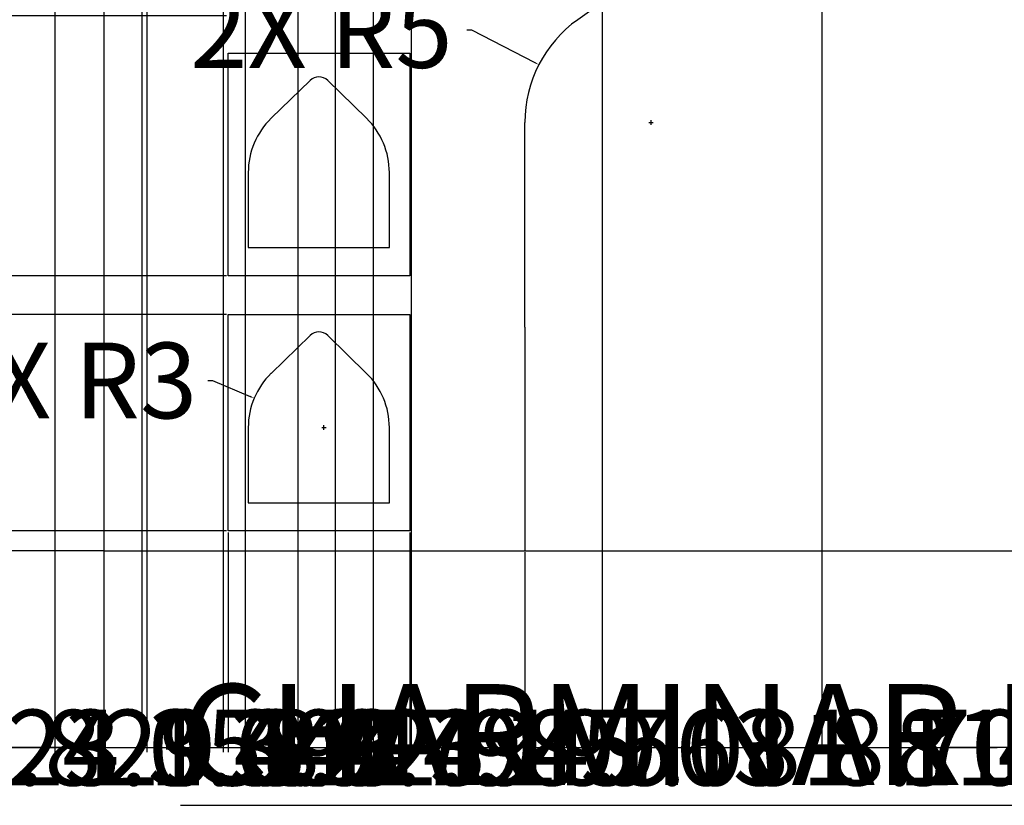
# Model space of a CAD drawing. Units: inches. Extents: x 168 to 318, y 152 to 314.
# Tile 2 of 7: x 201 to 240, y 152 to 183. Entities that reach past the tile are written whole.
import ezdxf

# ---------------------------------------------------------------- set-up
doc = ezdxf.new("R2010")
doc.units = ezdxf.units.IN
doc.header["$MEASUREMENT"] = 0
for name, color, linetype, lineweight in [('A-ANNO-DIMS', 2, 'Continuous', 18), ('A-ANNO-TEXT', 3, 'Continuous', 25), ('A-ELEV', 7, 'Continuous', 25)]:
    doc.layers.add(name, color=color, linetype=linetype, lineweight=lineweight)
doc.styles.get("Standard").update_dxf_attribs({"font": 'arial.ttf'})
doc.dimstyles.get("Standard").update_dxf_attribs({"dimtxt": 3, "dimasz": 0.18, "dimexe": 0.18, "dimexo": 0.0625, "dimgap": 0.09, "dimtad": 0, "dimtih": 1, "dimtoh": 1, "dimdec": 1, "dimzin": 0, "dimdsep": 46, "dimlunit": 3, "dimtxsty": 'Standard', "dimcen": 0.09, "dimadec": 0, "dimazin": 0, "dimtfac": 1, "dimtdec": 1, "dimtofl": 0, "dimtmove": 0, "dimatfit": 3, "dimfxl": 1, "dimtolj": 1, "dimtzin": 0, "dimarcsym": 0})

# ---------------------------------------------------------------- blocks, each defined once
blk = doc.blocks.new('NICHE-ARCHED')
for p, q in [((0.908, 5.124), (2.451, 6.627)), ((3.149, 6.626), (4.687, 5.124)), ((0, 2.975), (0, 0)), ((5.592, 0), (5.592, 2.977)), ((0, 0), (5.592, 0))]:
    blk.add_line(p, q)
for centre, radius, start, end in [((2.8, 6.268), 0.5, 45.6844, 134.2257), ((3, 2.975), 3, 134.2257, 180), ((2.592, 2.977), 3, 0, 45.6844)]:
    blk.add_arc(centre, radius, start, end)
blk = doc.blocks.new('*D29')
at = {"layer": 'A-ANNO-DIMS', "color": 0, "lineweight": -2, "ltscale": 0.2, "transparency": 16777216}
for p, q in [((184.724, 242.139), (184.724, 154.215)), ((299.445, 242.139), (299.445, 154.215)), ((184.904, 154.395), (235.924, 154.395)), ((299.265, 154.395), (248.245, 154.395))]:
    blk.add_line(p, q, dxfattribs=at)
at = {"layer": 'A-ANNO-DIMS', "color": 0, "ltscale": 0.2, "transparency": 16777216}
for points in [[(184.904, 154.425), (184.904, 154.365), (184.724, 154.395)], [(299.265, 154.425), (299.265, 154.365), (299.445, 154.395)]]:
    blk.add_solid(points, dxfattribs=at)
at = {"layer": 'Defpoints', "color": 0, "ltscale": 0.2, "transparency": 16777216}
for p in [(184.724, 242.201), (299.445, 242.201), (299.445, 154.395)]:
    blk.add_point(p, dxfattribs=at)
at = {"layer": 'A-ANNO-DIMS', "color": 0, "ltscale": 0.2, "transparency": 16777216, "insert": (242.084, 154.395), "char_height": 3, "attachment_point": 5}
blk.add_mtext('\\A1;114.72', dxfattribs=at)
blk = doc.blocks.new('*D48')
at = {"layer": 'A-ANNO-DIMS', "color": 0, "lineweight": -2, "ltscale": 0.2, "transparency": 16777216}
for p, q in [((192.404, 162.133), (192.404, 154.215)), ((204.404, 162.133), (204.404, 154.215)), ((192.584, 154.395), (196.322, 154.395)), ((204.224, 154.395), (200.487, 154.395))]:
    blk.add_line(p, q, dxfattribs=at)
at = {"layer": 'A-ANNO-DIMS', "color": 0, "ltscale": 0.2, "transparency": 16777216}
for points in [[(192.584, 154.425), (192.584, 154.365), (192.404, 154.395)], [(204.224, 154.425), (204.224, 154.365), (204.404, 154.395)]]:
    blk.add_solid(points, dxfattribs=at)
at = {"layer": 'Defpoints', "color": 0, "ltscale": 0.2, "transparency": 16777216}
for p in [(192.404, 162.195), (204.404, 162.195), (204.404, 154.395)]:
    blk.add_point(p, dxfattribs=at)
at = {"layer": 'A-ANNO-DIMS', "color": 0, "ltscale": 0.2, "transparency": 16777216, "insert": (198.404, 154.395), "char_height": 3, "attachment_point": 5}
blk.add_mtext('\\A1;12', dxfattribs=at)
blk = doc.blocks.new('*D49')
at = {"layer": 'A-ANNO-DIMS', "color": 0, "lineweight": -2, "ltscale": 0.2, "transparency": 16777216}
for p, q in [((209.325, 162.916), (209.325, 154.215)), ((204.404, 162.133), (204.404, 154.215)), ((204.584, 154.395), (209.145, 154.395)), ((209.325, 154.395), (209.505, 154.395))]:
    blk.add_line(p, q, dxfattribs=at)
at = {"layer": 'A-ANNO-DIMS', "color": 0, "ltscale": 0.2, "transparency": 16777216}
for points in [[(204.584, 154.425), (204.584, 154.365), (204.404, 154.395)], [(209.145, 154.425), (209.145, 154.365), (209.325, 154.395)]]:
    blk.add_solid(points, dxfattribs=at)
at = {"layer": 'Defpoints', "color": 0, "ltscale": 0.2, "transparency": 16777216}
for p in [(209.325, 162.979), (204.404, 162.195), (209.325, 154.395)]:
    blk.add_point(p, dxfattribs=at)
at = {"layer": 'A-ANNO-DIMS', "color": 0, "ltscale": 0.2, "transparency": 16777216, "insert": (213.536, 154.395), "char_height": 3, "attachment_point": 5}
blk.add_mtext('\\A1;4.92', dxfattribs=at)
blk = doc.blocks.new('*D50')
at = {"layer": 'A-ANNO-DIMS', "color": 0, "lineweight": -2, "ltscale": 0.2, "transparency": 16777216}
for p, q in [((209.325, 162.916), (209.325, 154.215)), ((216.522, 162.916), (216.522, 154.215)), ((209.505, 154.395), (216.342, 154.395)), ((216.522, 154.395), (216.702, 154.395))]:
    blk.add_line(p, q, dxfattribs=at)
at = {"layer": 'A-ANNO-DIMS', "color": 0, "ltscale": 0.2, "transparency": 16777216}
for points in [[(209.505, 154.425), (209.505, 154.365), (209.325, 154.395)], [(216.342, 154.425), (216.342, 154.365), (216.522, 154.395)]]:
    blk.add_solid(points, dxfattribs=at)
at = {"layer": 'Defpoints', "color": 0, "ltscale": 0.2, "transparency": 16777216}
for p in [(209.325, 162.979), (216.522, 162.979), (216.522, 154.395)]:
    blk.add_point(p, dxfattribs=at)
at = {"layer": 'A-ANNO-DIMS', "color": 0, "ltscale": 0.2, "transparency": 16777216, "insert": (221.841, 154.395), "char_height": 3, "attachment_point": 5}
blk.add_mtext('\\A1;7.197', dxfattribs=at)
blk = doc.blocks.new('*D51')
at = {"layer": 'A-ANNO-DIMS', "color": 0, "lineweight": -2, "ltscale": 0.2, "transparency": 16777216}
for p, q in [((216.522, 162.916), (216.522, 154.215)), ((221.084, 162.133), (221.084, 154.215)), ((216.702, 154.395), (220.904, 154.395)), ((221.084, 154.395), (221.264, 154.395))]:
    blk.add_line(p, q, dxfattribs=at)
at = {"layer": 'A-ANNO-DIMS', "color": 0, "ltscale": 0.2, "transparency": 16777216}
for points in [[(216.702, 154.425), (216.702, 154.365), (216.522, 154.395)], [(220.904, 154.425), (220.904, 154.365), (221.084, 154.395)]]:
    blk.add_solid(points, dxfattribs=at)
at = {"layer": 'Defpoints', "color": 0, "ltscale": 0.2, "transparency": 16777216}
for p in [(216.522, 162.979), (221.084, 162.195), (221.084, 154.395)]:
    blk.add_point(p, dxfattribs=at)
at = {"layer": 'A-ANNO-DIMS', "color": 0, "ltscale": 0.2, "transparency": 16777216, "insert": (226.477, 154.395), "char_height": 3, "attachment_point": 5}
blk.add_mtext('\\A1;4.563', dxfattribs=at)
blk = doc.blocks.new('*D52')
at = {"layer": 'A-ANNO-DIMS', "color": 0, "lineweight": -2, "ltscale": 0.2, "transparency": 16777216}
for p, q in [((221.084, 162.133), (221.084, 154.215)), ((263.084, 162.133), (263.084, 154.215)), ((221.264, 154.395), (239.801, 154.395)), ((262.904, 154.395), (244.368, 154.395))]:
    blk.add_line(p, q, dxfattribs=at)
at = {"layer": 'A-ANNO-DIMS', "color": 0, "ltscale": 0.2, "transparency": 16777216}
for points in [[(221.264, 154.425), (221.264, 154.365), (221.084, 154.395)], [(262.904, 154.425), (262.904, 154.365), (263.084, 154.395)]]:
    blk.add_solid(points, dxfattribs=at)
at = {"layer": 'Defpoints', "color": 0, "ltscale": 0.2, "transparency": 16777216}
for p in [(221.084, 162.195), (263.084, 162.195), (263.084, 154.395)]:
    blk.add_point(p, dxfattribs=at)
at = {"layer": 'A-ANNO-DIMS', "color": 0, "ltscale": 0.2, "transparency": 16777216, "insert": (242.084, 154.395), "char_height": 3, "attachment_point": 5}
blk.add_mtext('\\A1;42', dxfattribs=at)
blk = doc.blocks.new('*D58')
at = {"layer": 'A-ANNO-DIMS', "color": 0, "lineweight": -2, "ltscale": 0.2, "transparency": 16777216}
for p, q in [((176.881, 162.979), (176.881, 163.159)), ((176.881, 163.159), (177.061, 163.159)), ((209.262, 162.979), (176.701, 162.979)), ((176.881, 162.375), (176.881, 162.799)), ((204.342, 162.195), (176.701, 162.195))]:
    blk.add_line(p, q, dxfattribs=at)
at = {"layer": 'A-ANNO-DIMS', "color": 0, "ltscale": 0.2, "transparency": 16777216}
for points in [[(176.851, 162.799), (176.911, 162.799), (176.881, 162.979)], [(176.851, 162.375), (176.911, 162.375), (176.881, 162.195)]]:
    blk.add_solid(points, dxfattribs=at)
at = {"layer": 'Defpoints', "color": 0, "ltscale": 0.2, "transparency": 16777216}
for p in [(176.881, 162.979), (209.325, 162.979), (204.404, 162.195)]:
    blk.add_point(p, dxfattribs=at)
at = {"layer": 'A-ANNO-DIMS', "color": 0, "ltscale": 0.2, "transparency": 16777216, "insert": (181.05, 163.159), "char_height": 3, "attachment_point": 5}
blk.add_mtext('\\A1;0.78', dxfattribs=at)
blk = doc.blocks.new('*D59')
at = {"layer": 'A-ANNO-DIMS', "color": 0, "lineweight": -2, "ltscale": 0.2, "transparency": 16777216}
for p, q in [((209.262, 171.549), (176.701, 171.549)), ((176.881, 171.369), (176.881, 168.886)), ((176.881, 163.159), (176.881, 165.642)), ((209.262, 162.979), (176.701, 162.979))]:
    blk.add_line(p, q, dxfattribs=at)
at = {"layer": 'A-ANNO-DIMS', "color": 0, "ltscale": 0.2, "transparency": 16777216}
for points in [[(176.851, 171.369), (176.911, 171.369), (176.881, 171.549)], [(176.851, 163.159), (176.911, 163.159), (176.881, 162.979)]]:
    blk.add_solid(points, dxfattribs=at)
at = {"layer": 'Defpoints', "color": 0, "ltscale": 0.2, "transparency": 16777216}
for p in [(176.881, 171.549), (209.325, 171.549), (209.325, 162.979)]:
    blk.add_point(p, dxfattribs=at)
at = {"layer": 'A-ANNO-DIMS', "color": 0, "ltscale": 0.2, "transparency": 16777216, "insert": (176.881, 167.264), "char_height": 3, "attachment_point": 5}
blk.add_mtext('\\A1;8.57', dxfattribs=at)
blk = doc.blocks.new('*D60')
at = {"layer": 'A-ANNO-DIMS', "color": 0, "lineweight": -2, "ltscale": 0.2, "transparency": 16777216}
for p, q in [((176.881, 173.082), (176.881, 173.262)), ((176.881, 173.262), (177.061, 173.262)), ((209.262, 173.082), (176.701, 173.082)), ((176.881, 171.729), (176.881, 172.902)), ((209.262, 171.549), (176.701, 171.549))]:
    blk.add_line(p, q, dxfattribs=at)
at = {"layer": 'A-ANNO-DIMS', "color": 0, "ltscale": 0.2, "transparency": 16777216}
for points in [[(176.851, 172.902), (176.911, 172.902), (176.881, 173.082)], [(176.851, 171.729), (176.911, 171.729), (176.881, 171.549)]]:
    blk.add_solid(points, dxfattribs=at)
at = {"layer": 'Defpoints', "color": 0, "ltscale": 0.2, "transparency": 16777216}
for p in [(176.881, 173.082), (209.325, 173.082), (209.325, 171.549)]:
    blk.add_point(p, dxfattribs=at)
at = {"layer": 'A-ANNO-DIMS', "color": 0, "ltscale": 0.2, "transparency": 16777216, "insert": (180.906, 173.262), "char_height": 3, "attachment_point": 5}
blk.add_mtext('\\A1;1.53', dxfattribs=at)
blk = doc.blocks.new('*D61')
at = {"layer": 'A-ANNO-DIMS', "color": 0, "lineweight": -2, "ltscale": 0.2, "transparency": 16777216}
for p, q in [((209.262, 183.379), (176.701, 183.379)), ((176.881, 183.199), (176.881, 179.852)), ((176.881, 173.262), (176.881, 176.609)), ((209.262, 173.082), (176.701, 173.082))]:
    blk.add_line(p, q, dxfattribs=at)
at = {"layer": 'A-ANNO-DIMS', "color": 0, "ltscale": 0.2, "transparency": 16777216}
for points in [[(176.851, 183.199), (176.911, 183.199), (176.881, 183.379)], [(176.851, 173.262), (176.911, 173.262), (176.881, 173.082)]]:
    blk.add_solid(points, dxfattribs=at)
at = {"layer": 'Defpoints', "color": 0, "ltscale": 0.2, "transparency": 16777216}
for p in [(176.881, 183.379), (209.325, 183.379), (209.325, 173.082)]:
    blk.add_point(p, dxfattribs=at)
at = {"layer": 'A-ANNO-DIMS', "color": 0, "ltscale": 0.2, "transparency": 16777216, "insert": (176.881, 178.231), "char_height": 3, "attachment_point": 5}
blk.add_mtext('\\A1;10.296', dxfattribs=at)
blk = doc.blocks.new('*D70')
at = {"layer": 'A-ANNO-DIMS', "color": 0, "lineweight": -2, "ltscale": 0.2, "transparency": 16777216}
for p, q in [((190.252, 205.813), (190.252, 154.215)), ((194.576, 205.813), (194.576, 154.215)), ((190.432, 154.395), (194.396, 154.395)), ((194.576, 154.395), (194.756, 154.395))]:
    blk.add_line(p, q, dxfattribs=at)
at = {"layer": 'A-ANNO-DIMS', "color": 0, "ltscale": 0.2, "transparency": 16777216}
for points in [[(190.432, 154.425), (190.432, 154.365), (190.252, 154.395)], [(194.396, 154.425), (194.396, 154.365), (194.576, 154.395)]]:
    blk.add_solid(points, dxfattribs=at)
at = {"layer": 'Defpoints', "color": 0, "ltscale": 0.2, "transparency": 16777216}
for p in [(190.252, 205.875), (194.576, 205.875), (194.576, 154.395)]:
    blk.add_point(p, dxfattribs=at)
at = {"layer": 'A-ANNO-DIMS', "color": 0, "ltscale": 0.2, "transparency": 16777216, "insert": (199.968, 154.395), "char_height": 3, "attachment_point": 5}
blk.add_mtext('\\A1;4.323', dxfattribs=at)
blk = doc.blocks.new('*D71')
at = {"layer": 'A-ANNO-DIMS', "color": 0, "lineweight": -2, "ltscale": 0.2, "transparency": 16777216}
for p, q in [((194.576, 205.813), (194.576, 154.215)), ((198.404, 205.813), (198.404, 154.215)), ((194.756, 154.395), (198.224, 154.395)), ((198.404, 154.395), (198.584, 154.395))]:
    blk.add_line(p, q, dxfattribs=at)
at = {"layer": 'A-ANNO-DIMS', "color": 0, "ltscale": 0.2, "transparency": 16777216}
for points in [[(194.756, 154.425), (194.756, 154.365), (194.576, 154.395)], [(198.224, 154.425), (198.224, 154.365), (198.404, 154.395)]]:
    blk.add_solid(points, dxfattribs=at)
at = {"layer": 'Defpoints', "color": 0, "ltscale": 0.2, "transparency": 16777216}
for p in [(194.576, 205.875), (198.404, 205.875), (198.404, 154.395)]:
    blk.add_point(p, dxfattribs=at)
at = {"layer": 'A-ANNO-DIMS', "color": 0, "ltscale": 0.2, "transparency": 16777216, "insert": (203.738, 154.395), "char_height": 3, "attachment_point": 5}
blk.add_mtext('\\A1;3.829', dxfattribs=at)
blk = doc.blocks.new('*D72')
at = {"layer": 'A-ANNO-DIMS', "color": 0, "lineweight": -2, "ltscale": 0.2, "transparency": 16777216}
for p, q in [((198.404, 205.813), (198.404, 154.215)), ((202.463, 205.813), (202.463, 154.215)), ((198.584, 154.395), (202.283, 154.395)), ((202.463, 154.395), (202.643, 154.395))]:
    blk.add_line(p, q, dxfattribs=at)
at = {"layer": 'A-ANNO-DIMS', "color": 0, "ltscale": 0.2, "transparency": 16777216}
for points in [[(198.584, 154.425), (198.584, 154.365), (198.404, 154.395)], [(202.283, 154.425), (202.283, 154.365), (202.463, 154.395)]]:
    blk.add_solid(points, dxfattribs=at)
at = {"layer": 'Defpoints', "color": 0, "ltscale": 0.2, "transparency": 16777216}
for p in [(198.404, 205.875), (202.463, 205.875), (202.463, 154.395)]:
    blk.add_point(p, dxfattribs=at)
at = {"layer": 'A-ANNO-DIMS', "color": 0, "ltscale": 0.2, "transparency": 16777216, "insert": (207.858, 154.395), "char_height": 3, "attachment_point": 5}
blk.add_mtext('\\A1;4.058', dxfattribs=at)
blk = doc.blocks.new('*D73')
at = {"layer": 'A-ANNO-DIMS', "color": 0, "lineweight": -2, "ltscale": 0.2, "transparency": 16777216}
for p, q in [((202.463, 205.813), (202.463, 154.215)), ((205.91, 205.813), (205.91, 154.215)), ((202.643, 154.395), (205.73, 154.395)), ((205.91, 154.395), (206.09, 154.395))]:
    blk.add_line(p, q, dxfattribs=at)
at = {"layer": 'A-ANNO-DIMS', "color": 0, "ltscale": 0.2, "transparency": 16777216}
for points in [[(202.643, 154.425), (202.643, 154.365), (202.463, 154.395)], [(205.73, 154.425), (205.73, 154.365), (205.91, 154.395)]]:
    blk.add_solid(points, dxfattribs=at)
at = {"layer": 'Defpoints', "color": 0, "ltscale": 0.2, "transparency": 16777216}
for p in [(202.463, 205.875), (205.91, 205.875), (205.91, 154.395)]:
    blk.add_point(p, dxfattribs=at)
at = {"layer": 'A-ANNO-DIMS', "color": 0, "ltscale": 0.2, "transparency": 16777216, "insert": (211.24, 154.395), "char_height": 3, "attachment_point": 5}
blk.add_mtext('\\A1;3.447', dxfattribs=at)
blk = doc.blocks.new('*D74')
at = {"layer": 'A-ANNO-DIMS', "color": 0, "lineweight": -2, "ltscale": 0.2, "transparency": 16777216}
for p, q in [((205.91, 205.813), (205.91, 154.215)), ((209.123, 205.813), (209.123, 154.215)), ((206.09, 154.395), (208.943, 154.395)), ((209.123, 154.395), (209.303, 154.395))]:
    blk.add_line(p, q, dxfattribs=at)
at = {"layer": 'A-ANNO-DIMS', "color": 0, "ltscale": 0.2, "transparency": 16777216}
for points in [[(206.09, 154.425), (206.09, 154.365), (205.91, 154.395)], [(208.943, 154.425), (208.943, 154.365), (209.123, 154.395)]]:
    blk.add_solid(points, dxfattribs=at)
at = {"layer": 'Defpoints', "color": 0, "ltscale": 0.2, "transparency": 16777216}
for p in [(205.91, 205.875), (209.123, 205.875), (209.123, 154.395)]:
    blk.add_point(p, dxfattribs=at)
at = {"layer": 'A-ANNO-DIMS', "color": 0, "ltscale": 0.2, "transparency": 16777216, "insert": (214.453, 154.395), "char_height": 3, "attachment_point": 5}
blk.add_mtext('\\A1;3.213', dxfattribs=at)
blk = doc.blocks.new('*D84')
at = {"layer": 'A-ANNO-DIMS', "color": 0, "lineweight": -2, "ltscale": 0.2, "transparency": 16777216}
for p, q in [((206.099, 227.876), (206.099, 154.215)), ((204.404, 227.113), (204.404, 154.215)), ((204.584, 154.395), (205.919, 154.395)), ((206.099, 154.395), (206.279, 154.395))]:
    blk.add_line(p, q, dxfattribs=at)
at = {"layer": 'A-ANNO-DIMS', "color": 0, "ltscale": 0.2, "transparency": 16777216}
for points in [[(204.584, 154.425), (204.584, 154.365), (204.404, 154.395)], [(205.919, 154.425), (205.919, 154.365), (206.099, 154.395)]]:
    blk.add_solid(points, dxfattribs=at)
at = {"layer": 'Defpoints', "color": 0, "ltscale": 0.2, "transparency": 16777216}
for p in [(206.099, 227.938), (204.404, 227.175), (206.099, 154.395)]:
    blk.add_point(p, dxfattribs=at)
at = {"layer": 'A-ANNO-DIMS', "color": 0, "ltscale": 0.2, "transparency": 16777216, "insert": (211.283, 154.395), "char_height": 3, "attachment_point": 5}
blk.add_mtext('\\A1;1.694', dxfattribs=at)
blk = doc.blocks.new('*D85')
at = {"layer": 'A-ANNO-DIMS', "color": 0, "lineweight": -2, "ltscale": 0.2, "transparency": 16777216}
for p, q in [((206.099, 227.876), (206.099, 154.215)), ((209.999, 227.876), (209.999, 154.215)), ((206.279, 154.395), (209.819, 154.395)), ((209.999, 154.395), (210.179, 154.395))]:
    blk.add_line(p, q, dxfattribs=at)
at = {"layer": 'A-ANNO-DIMS', "color": 0, "ltscale": 0.2, "transparency": 16777216}
for points in [[(206.279, 154.425), (206.279, 154.365), (206.099, 154.395)], [(209.819, 154.425), (209.819, 154.365), (209.999, 154.395)]]:
    blk.add_solid(points, dxfattribs=at)
at = {"layer": 'Defpoints', "color": 0, "ltscale": 0.2, "transparency": 16777216}
for p in [(206.099, 227.938), (209.999, 227.938), (209.999, 154.395)]:
    blk.add_point(p, dxfattribs=at)
at = {"layer": 'A-ANNO-DIMS', "color": 0, "ltscale": 0.2, "transparency": 16777216, "insert": (213.002, 154.395), "char_height": 3, "attachment_point": 5}
blk.add_mtext('\\A1;3.9', dxfattribs=at)
blk = doc.blocks.new('*D86')
at = {"layer": 'A-ANNO-DIMS', "color": 0, "lineweight": -2, "ltscale": 0.2, "transparency": 16777216}
for p, q in [((212.084, 220.813), (212.084, 154.215)), ((213.573, 220.813), (213.573, 154.215)), ((212.264, 154.395), (213.393, 154.395)), ((213.573, 154.395), (213.753, 154.395))]:
    blk.add_line(p, q, dxfattribs=at)
at = {"layer": 'A-ANNO-DIMS', "color": 0, "ltscale": 0.2, "transparency": 16777216}
for points in [[(212.264, 154.425), (212.264, 154.365), (212.084, 154.395)], [(213.393, 154.425), (213.393, 154.365), (213.573, 154.395)]]:
    blk.add_solid(points, dxfattribs=at)
at = {"layer": 'Defpoints', "color": 0, "ltscale": 0.2, "transparency": 16777216}
for p in [(212.084, 220.875), (213.573, 220.875), (213.573, 154.395)]:
    blk.add_point(p, dxfattribs=at)
at = {"layer": 'A-ANNO-DIMS', "color": 0, "ltscale": 0.2, "transparency": 16777216, "insert": (217.601, 154.395), "char_height": 3, "attachment_point": 5}
blk.add_mtext('\\A1;1.49', dxfattribs=at)
blk = doc.blocks.new('*D87')
at = {"layer": 'A-ANNO-DIMS', "color": 0, "lineweight": -2, "ltscale": 0.2, "transparency": 16777216}
for p, q in [((213.573, 220.813), (213.573, 154.215)), ((216.573, 220.813), (216.573, 154.215)), ((213.753, 154.395), (214.001, 154.395)), ((216.393, 154.395), (216.145, 154.395))]:
    blk.add_line(p, q, dxfattribs=at)
at = {"layer": 'A-ANNO-DIMS', "color": 0, "ltscale": 0.2, "transparency": 16777216}
for points in [[(213.753, 154.425), (213.753, 154.365), (213.573, 154.395)], [(216.393, 154.425), (216.393, 154.365), (216.573, 154.395)]]:
    blk.add_solid(points, dxfattribs=at)
at = {"layer": 'Defpoints', "color": 0, "ltscale": 0.2, "transparency": 16777216}
for p in [(213.573, 220.875), (216.573, 220.875), (216.573, 154.395)]:
    blk.add_point(p, dxfattribs=at)
at = {"layer": 'A-ANNO-DIMS', "color": 0, "ltscale": 0.2, "transparency": 16777216, "insert": (215.073, 154.395), "char_height": 3, "attachment_point": 5}
blk.add_mtext('\\A1;3', dxfattribs=at)
blk = doc.blocks.new('*D88')
at = {"layer": 'A-ANNO-DIMS', "color": 0, "lineweight": -2, "ltscale": 0.2, "transparency": 16777216}
for p, q in [((212.084, 207.331), (212.084, 154.215)), ((215.07, 207.331), (215.07, 154.215)), ((212.264, 154.395), (214.89, 154.395)), ((215.07, 154.395), (215.25, 154.395))]:
    blk.add_line(p, q, dxfattribs=at)
at = {"layer": 'A-ANNO-DIMS', "color": 0, "ltscale": 0.2, "transparency": 16777216}
for points in [[(212.264, 154.425), (212.264, 154.365), (212.084, 154.395)], [(214.89, 154.425), (214.89, 154.365), (215.07, 154.395)]]:
    blk.add_solid(points, dxfattribs=at)
at = {"layer": 'Defpoints', "color": 0, "ltscale": 0.2, "transparency": 16777216}
for p in [(212.084, 207.394), (215.07, 207.394), (215.07, 154.395)]:
    blk.add_point(p, dxfattribs=at)
at = {"layer": 'A-ANNO-DIMS', "color": 0, "ltscale": 0.2, "transparency": 16777216, "insert": (220.438, 154.395), "char_height": 3, "attachment_point": 5}
blk.add_mtext('\\A1;2.985', dxfattribs=at)
blk = doc.blocks.new('*D89')
at = {"layer": 'A-ANNO-DIMS', "color": 0, "lineweight": -2, "ltscale": 0.2, "transparency": 16777216}
for p, q in [((215.07, 207.331), (215.07, 154.215)), ((224.151, 207.331), (224.151, 154.215)), ((215.25, 154.395), (223.971, 154.395)), ((224.151, 154.395), (224.331, 154.395))]:
    blk.add_line(p, q, dxfattribs=at)
at = {"layer": 'A-ANNO-DIMS', "color": 0, "ltscale": 0.2, "transparency": 16777216}
for points in [[(215.25, 154.425), (215.25, 154.365), (215.07, 154.395)], [(223.971, 154.425), (223.971, 154.365), (224.151, 154.395)]]:
    blk.add_solid(points, dxfattribs=at)
at = {"layer": 'Defpoints', "color": 0, "ltscale": 0.2, "transparency": 16777216}
for p in [(215.07, 207.394), (224.151, 207.394), (224.151, 154.395)]:
    blk.add_point(p, dxfattribs=at)
at = {"layer": 'A-ANNO-DIMS', "color": 0, "ltscale": 0.2, "transparency": 16777216, "insert": (229.193, 154.395), "char_height": 3, "attachment_point": 5}
blk.add_mtext('\\A1;9.081', dxfattribs=at)
blk = doc.blocks.new('*D90')
at = {"layer": 'A-ANNO-DIMS', "color": 0, "lineweight": -2, "ltscale": 0.2, "transparency": 16777216}
for p, q in [((224.151, 207.331), (224.151, 154.215)), ((232.855, 207.331), (232.855, 154.215)), ((224.331, 154.395), (232.675, 154.395)), ((232.855, 154.395), (233.035, 154.395))]:
    blk.add_line(p, q, dxfattribs=at)
at = {"layer": 'A-ANNO-DIMS', "color": 0, "ltscale": 0.2, "transparency": 16777216}
for points in [[(224.331, 154.425), (224.331, 154.365), (224.151, 154.395)], [(232.675, 154.425), (232.675, 154.365), (232.855, 154.395)]]:
    blk.add_solid(points, dxfattribs=at)
at = {"layer": 'Defpoints', "color": 0, "ltscale": 0.2, "transparency": 16777216}
for p in [(224.151, 207.394), (232.855, 207.394), (232.855, 154.395)]:
    blk.add_point(p, dxfattribs=at)
at = {"layer": 'A-ANNO-DIMS', "color": 0, "ltscale": 0.2, "transparency": 16777216, "insert": (238.2, 154.395), "char_height": 3, "attachment_point": 5}
blk.add_mtext('\\A1;8.705', dxfattribs=at)
blk = doc.blocks.new('*D91')
at = {"layer": 'A-ANNO-DIMS', "color": 0, "lineweight": -2, "ltscale": 0.2, "transparency": 16777216}
for p, q in [((232.855, 207.331), (232.855, 154.215)), ((240.855, 207.331), (240.855, 154.215)), ((233.035, 154.395), (235.777, 154.395)), ((240.675, 154.395), (237.934, 154.395))]:
    blk.add_line(p, q, dxfattribs=at)
at = {"layer": 'A-ANNO-DIMS', "color": 0, "ltscale": 0.2, "transparency": 16777216}
for points in [[(233.035, 154.425), (233.035, 154.365), (232.855, 154.395)], [(240.675, 154.425), (240.675, 154.365), (240.855, 154.395)]]:
    blk.add_solid(points, dxfattribs=at)
at = {"layer": 'Defpoints', "color": 0, "ltscale": 0.2, "transparency": 16777216}
for p in [(232.855, 207.394), (240.855, 207.394), (240.855, 154.395)]:
    blk.add_point(p, dxfattribs=at)
at = {"layer": 'A-ANNO-DIMS', "color": 0, "ltscale": 0.2, "transparency": 16777216, "insert": (236.855, 154.395), "char_height": 3, "attachment_point": 5}
blk.add_mtext('\\A1;8', dxfattribs=at)
blk = doc.blocks.new('*D97')
at = {"layer": 'A-ANNO-DIMS', "color": 0, "lineweight": -2, "ltscale": 0.2, "transparency": 16777216}
for p, q in [((218.791, 182.822), (218.971, 182.822)), ((218.971, 182.822), (221.479, 181.532)), ((225.994, 179.161), (226.174, 179.161)), ((226.084, 179.071), (226.084, 179.251))]:
    blk.add_line(p, q, dxfattribs=at)
at = {"layer": 'A-ANNO-DIMS', "color": 0, "ltscale": 0.2, "transparency": 16777216}
blk.add_solid([(221.492, 181.558), (221.465, 181.505), (221.639, 181.449)], dxfattribs=at)
at = {"layer": 'Defpoints', "color": 0, "ltscale": 0.2, "transparency": 16777216}
for p in [(221.639, 181.449), (226.084, 179.161)]:
    blk.add_point(p, dxfattribs=at)
at = {"layer": 'A-ANNO-DIMS', "color": 0, "ltscale": 0.2, "transparency": 16777216, "insert": (213.023, 182.822), "char_height": 3, "attachment_point": 5}
blk.add_mtext('\\A1;2X R5', dxfattribs=at)
blk = doc.blocks.new('*D100')
at = {"layer": 'A-ANNO-DIMS', "color": 0, "lineweight": -2, "ltscale": 0.2, "transparency": 16777216}
for p, q in [((208.521, 168.938), (208.701, 168.938)), ((208.701, 168.938), (210.193, 168.308)), ((213.033, 167.072), (213.213, 167.072)), ((213.123, 166.982), (213.123, 167.162))]:
    blk.add_line(p, q, dxfattribs=at)
at = {"layer": 'A-ANNO-DIMS', "color": 0, "ltscale": 0.2, "transparency": 16777216}
blk.add_solid([(210.205, 168.336), (210.182, 168.28), (210.359, 168.238)], dxfattribs=at)
at = {"layer": 'Defpoints', "color": 0, "ltscale": 0.2, "transparency": 16777216}
for p in [(210.359, 168.238), (213.123, 167.072)]:
    blk.add_point(p, dxfattribs=at)
at = {"layer": 'A-ANNO-DIMS', "color": 0, "ltscale": 0.2, "transparency": 16777216, "insert": (201.765, 168.938), "char_height": 3, "attachment_point": 5}
blk.add_mtext('\\A1;16X R3', dxfattribs=at)

msp = doc.modelspace()

# ---------------------------------------------------------------- linework, layer by layer
at = {"layer": 'A-ELEV'}
for p, q in [((204.4044, 198.1954), (204.4044, 162.1954)), ((239.1785, 194.6573), (223.1785, 183.2299)), ((221.0845, 171.0451), (221.0845, 179.1611)), ((221.0845, 171.0451), (221.0845, 162.1954)), ((204.4044, 162.1954), (192.4044, 162.1954)), ((204.4044, 162.1954), (279.7645, 162.1954))]:
    msp.add_line(p, q, dxfattribs=at)
for points in [[(209.3248, 181.9003), (216.5216, 181.9003), (216.5216, 173.0824), (209.3248, 173.0824)], [(209.3248, 171.5491), (216.5216, 171.5491), (216.5216, 162.9789), (209.3248, 162.9789)]]:
    msp.add_lwpolyline(points, close=True, dxfattribs=at)
msp.add_arc((226.0845, 179.1611), 5, 125.53477, 180, dxfattribs=at)

# ---------------------------------------------------------------- block references
for p in [(210.123, 174.2005), (210.123, 164.097)]:
    msp.add_blockref('NICHE-ARCHED', p, dxfattribs=at)

# ---------------------------------------------------------------- texts
at = {"layer": 'A-ANNO-TEXT', "ltscale": 0.2, "insert": (207.4369, 156.91), "char_height": 4, "attachment_point": 1}
msp.add_mtext_dynamic_manual_height_columns('{\\fArial|b1|i0|c0|p34;\\LCHARMINAR ELEVATION }', width=92.221498, gutter_width=1, heights=[0], dxfattribs=at)

# ---------------------------------------------------------------- dimensions: what is measured, and where the dimension line sits
at = {"layer": 'A-ANNO-DIMS', "ltscale": 0.2}
for base, p1, p2, override, picture, middle in [((299.4446, 154.3954), (184.7244, 242.2013), (299.4446, 242.2013), {"dimdec": 2, "dimlfac": 1, "dimrnd": 0, "dimzin": 0, "dimdsep": 46, "dimlunit": 2}, '*D29', (242.0845, 154.3954)), ((206.0986, 154.3954), (204.4044, 227.1751), (206.0986, 227.9381), {"dimdec": 3, "dimlfac": 1, "dimrnd": 0, "dimzin": 0, "dimdsep": 46, "dimlunit": 2}, '*D84', (211.283, 154.3954)), ((209.9986, 154.3954), (206.0986, 227.9381), (209.9986, 227.9381), {"dimdec": 1, "dimlfac": 1, "dimrnd": 0, "dimzin": 0, "dimdsep": 46, "dimlunit": 2}, '*D85', (213.0015, 154.3954)), ((213.5729, 154.3954), (212.0845, 220.8755), (213.5729, 220.8755), {"dimdec": 2, "dimlfac": 1, "dimrnd": 0, "dimzin": 0, "dimdsep": 46, "dimlunit": 2}, '*D86', (217.601, 154.3954)), ((216.5729, 154.3954), (213.5729, 220.8755), (216.5729, 220.8755), {"dimdec": 0, "dimlfac": 1, "dimrnd": 0, "dimzin": 0, "dimdsep": 46, "dimlunit": 2}, '*D87', (215.0729, 154.3954)), ((215.0696, 154.3954), (212.0845, 207.3935), (215.0696, 207.3935), {"dimdec": 3, "dimlfac": 1, "dimrnd": 0, "dimzin": 0, "dimdsep": 46, "dimlunit": 2}, '*D88', (220.4382, 154.3954)), ((224.1506, 154.3954), (215.0696, 207.3935), (224.1506, 207.3935), {"dimdec": 3, "dimlfac": 1, "dimrnd": 0, "dimzin": 0, "dimdsep": 46, "dimlunit": 2}, '*D89', (229.1928, 154.3954)), ((232.8554, 154.3954), (224.1506, 207.3935), (232.8554, 207.3935), {"dimdec": 3, "dimlfac": 1, "dimrnd": 0, "dimzin": 0, "dimdsep": 46, "dimlunit": 2}, '*D90', (238.2004, 154.3954)), ((240.8554, 154.3954), (232.8554, 207.3935), (240.8554, 207.3935), {"dimdec": 0, "dimlfac": 1, "dimrnd": 0, "dimzin": 0, "dimdsep": 46, "dimlunit": 2}, '*D91', (236.8554, 154.3954)), ((194.5757, 154.3954), (190.2524, 205.8755), (194.5757, 205.8755), {"dimdec": 3, "dimlfac": 1, "dimrnd": 0, "dimzin": 0, "dimdsep": 46, "dimlunit": 2}, '*D70', (199.9678, 154.3954)), ((198.4044, 154.3954), (194.5757, 205.8755), (198.4044, 205.8755), {"dimdec": 3, "dimlfac": 1, "dimrnd": 0, "dimzin": 0, "dimdsep": 46, "dimlunit": 2}, '*D71', (203.7382, 154.3954)), ((202.4627, 154.3954), (198.4044, 205.8755), (202.4627, 205.8755), {"dimdec": 3, "dimlfac": 1, "dimrnd": 0, "dimzin": 0, "dimdsep": 46, "dimlunit": 2}, '*D72', (207.8578, 154.3954)), ((205.9096, 154.3954), (202.4627, 205.8755), (205.9096, 205.8755), {"dimdec": 3, "dimlfac": 1, "dimrnd": 0, "dimzin": 0, "dimdsep": 46, "dimlunit": 2}, '*D73', (211.2403, 154.3954)), ((209.1228, 154.3954), (205.9096, 205.8755), (209.1228, 205.8755), {"dimdec": 3, "dimlfac": 1, "dimrnd": 0, "dimzin": 0, "dimdsep": 46, "dimlunit": 2}, '*D74', (214.4535, 154.3954)), ((209.3248, 154.3954), (204.4044, 162.1954), (209.3248, 162.9789), {"dimdec": 2, "dimlfac": 1, "dimrnd": 0, "dimzin": 0, "dimdsep": 46, "dimlunit": 2}, '*D49', (213.5362, 154.3954)), ((216.5216, 154.3954), (209.3248, 162.9789), (216.5216, 162.9789), {"dimdec": 3, "dimlfac": 1, "dimrnd": 0, "dimzin": 0, "dimdsep": 46, "dimlunit": 2}, '*D50', (221.8411, 154.3954)), ((221.0845, 154.3954), (216.5216, 162.9789), (221.0845, 162.1954), {"dimdec": 3, "dimlfac": 1, "dimrnd": 0, "dimzin": 0, "dimdsep": 46, "dimlunit": 2}, '*D51', (226.4766, 154.3954)), ((204.4044, 154.3954), (192.4044, 162.1954), (204.4044, 162.1954), {"dimdec": 0, "dimlfac": 1, "dimrnd": 0, "dimzin": 0, "dimdsep": 46, "dimlunit": 2}, '*D48', (198.4044, 154.3954)), ((263.0845, 154.3954), (221.0845, 162.1954), (263.0845, 162.1954), {"dimdec": 0, "dimlfac": 1, "dimrnd": 0, "dimzin": 0, "dimdsep": 46, "dimlunit": 2}, '*D52', (242.0845, 154.3954))]:
    dim = msp.add_linear_dim(base=base, p1=p1, p2=p2, dimstyle='Standard', override=override, dxfattribs=at)
    dim.commit()
    dim.dimension.update_dxf_attribs({"geometry": picture, "text_midpoint": middle})
for center, mpoint, text, picture, middle in [((226.0845, 179.1611), (221.6387, 181.4492), '2X <>', '*D97', (213.0225, 182.822)), ((213.1231, 167.0717), (210.3591, 168.238), '16X <>', '*D100', (201.7646, 168.9377))]:
    dim = msp.add_radius_dim(center=center, mpoint=mpoint, text=text, dimstyle='Standard', override={"dimdec": 0, "dimlfac": 1, "dimrnd": 0, "dimzin": 0, "dimdsep": 46, "dimlunit": 2}, dxfattribs=at)
    dim.commit()
    dim.dimension.update_dxf_attribs({"geometry": picture, "text_midpoint": middle, "dimtype": 164})
for base, p1, p2, override, picture, middle in [((176.8805, 183.3788), (209.3248, 173.0824), (209.3248, 183.3788), {"dimdec": 3, "dimlfac": 1, "dimrnd": 0, "dimzin": 0, "dimdsep": 46, "dimlunit": 2}, '*D61', (176.8805, 178.2306)), ((176.8805, 173.0824), (209.3248, 171.5491), (209.3248, 173.0824), {"dimdec": 2, "dimlfac": 1, "dimrnd": 0, "dimzin": 0, "dimdsep": 46, "dimlunit": 2}, '*D60', (180.9056, 173.2624)), ((176.8805, 171.5491), (209.3248, 162.9789), (209.3248, 171.5491), {"dimdec": 2, "dimlfac": 1, "dimrnd": 0, "dimzin": 0, "dimdsep": 46, "dimlunit": 2}, '*D59', (176.8805, 167.264)), ((176.8805, 162.9789), (204.4044, 162.1954), (209.3248, 162.9789), {"dimdec": 2, "dimlfac": 1, "dimrnd": 0, "dimzin": 0, "dimdsep": 46, "dimlunit": 2}, '*D58', (181.0499, 163.1589))]:
    dim = msp.add_linear_dim(base=base, p1=p1, p2=p2, angle=90, dimstyle='Standard', override=override, dxfattribs=at)
    dim.commit()
    dim.dimension.update_dxf_attribs({"geometry": picture, "text_midpoint": middle})

doc.saveas('drawing.dxf')
